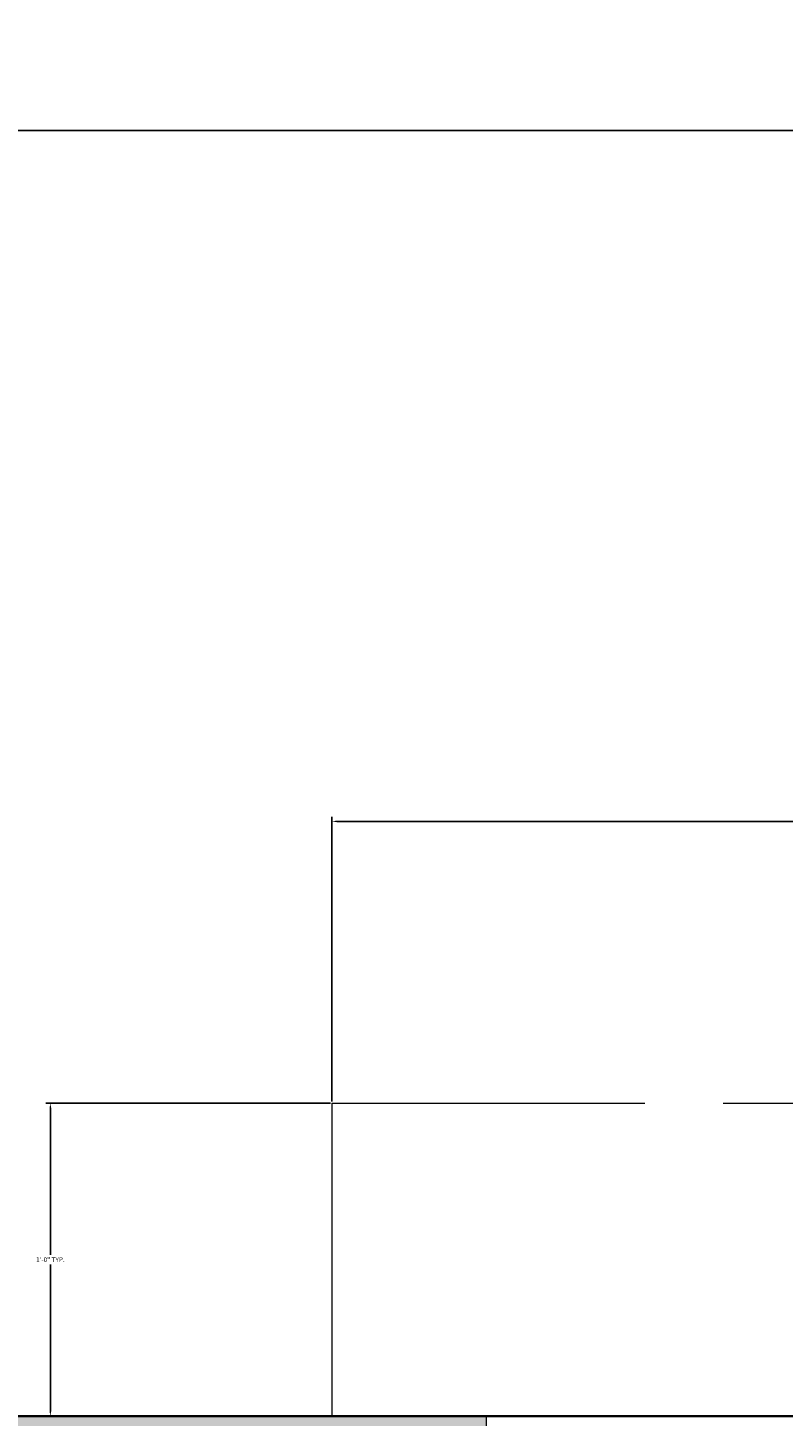
# Model space of a CAD drawing. Units: inches. Extents: x -5 to 482, y -460 to 66.
# Tile 27 of 31: x 48 to 77, y 13 to 66. Entities that reach past the tile are written whole.
import ezdxf

# ---------------------------------------------------------------- set-up
doc = ezdxf.new("R2010")
doc.units = ezdxf.units.IN
doc.header["$MEASUREMENT"] = 0
doc.linetypes.add('ACAD_ISO02W100', pattern=[15, 12, -3])
for name, color, linetype, lineweight in [('A-ANNO-DIMS', 2, 'Continuous', 18), ('A-GLAZ', 4, 'Continuous', 18), ('A-GLAZ-OVHD', 4, 'ACAD_ISO02W100', 13), ('A-WALL', 7, 'Continuous', 35), ('A-WALL-PATT', 152, 'Continuous', 13)]:
    doc.layers.add(name, color=color, linetype=linetype, lineweight=lineweight)
doc.styles.get("Standard").update_dxf_attribs({"font": 'arial.ttf'})
doc.dimstyles.get("Standard").update_dxf_attribs({"dimtxt": 0.18, "dimasz": 0.18, "dimexe": 0.18, "dimexo": 0.0625, "dimgap": 0.09, "dimtad": 0, "dimtih": 1, "dimtoh": 1, "dimdec": 0, "dimzin": 0, "dimdsep": 46, "dimlunit": 3, "dimtxsty": 'Standard', "dimcen": 0.09, "dimadec": 0, "dimazin": 0, "dimtfac": 1, "dimtdec": 0, "dimtofl": 0, "dimtmove": 0, "dimatfit": 3, "dimfxl": 1, "dimtolj": 1, "dimtzin": 0, "dimarcsym": 0})

# ---------------------------------------------------------------- blocks, each defined once
blk = doc.blocks.new('*D3')
at = {"layer": 'A-ANNO-DIMS', "color": 0, "lineweight": -2, "transparency": 16777216}
for p, q in [((32.877, 13.214), (32.877, 62.612)), ((33.057, 62.432), (221.233, 62.432)), ((430.197, 62.432), (242.02, 62.432)), ((430.377, 13.214), (430.377, 62.612))]:
    blk.add_line(p, q, dxfattribs=at)
at = {"layer": 'A-ANNO-DIMS', "color": 0, "transparency": 16777216}
for points in [[(33.057, 62.462), (33.057, 62.402), (32.877, 62.432)], [(430.197, 62.462), (430.197, 62.402), (430.377, 62.432)]]:
    blk.add_solid(points, dxfattribs=at)
at = {"layer": 'Defpoints', "color": 0, "transparency": 16777216}
for p in [(430.377, 62.432), (32.877, 13.151), (430.377, 13.151)]:
    blk.add_point(p, dxfattribs=at)
at = {"layer": 'A-ANNO-DIMS', "color": 0, "transparency": 16777216, "insert": (231.627, 62.432), "char_height": 6, "attachment_point": 5}
blk.add_mtext('\\A1;33\'-2"', dxfattribs=at)
blk = doc.blocks.new('WIN-SHADE-72IN')
for q in [(72, 12), (0, 0)]:
    blk.add_line((0, 12), q)
blk = doc.blocks.new('*D45')
at = {"layer": 'A-ANNO-DIMS', "color": 0, "lineweight": -2, "transparency": 16777216}
for p, q in [((59.948, 25.214), (59.948, 36.131)), ((60.128, 35.951), (94.251, 35.951)), ((131.768, 35.951), (97.645, 35.951)), ((131.948, 25.214), (131.948, 36.131))]:
    blk.add_line(p, q, dxfattribs=at)
at = {"layer": 'A-ANNO-DIMS', "color": 0, "transparency": 16777216}
for points in [[(60.128, 35.981), (60.128, 35.921), (59.948, 35.951)], [(131.768, 35.981), (131.768, 35.921), (131.948, 35.951)]]:
    blk.add_solid(points, dxfattribs=at)
at = {"layer": 'Defpoints', "color": 0, "transparency": 16777216}
for p in [(131.948, 35.951), (59.948, 25.151), (131.948, 25.151)]:
    blk.add_point(p, dxfattribs=at)
at = {"layer": 'A-ANNO-DIMS', "color": 0, "transparency": 16777216, "insert": (95.948, 35.951), "char_height": 0.18, "attachment_point": 5}
blk.add_mtext('\\A1;WINDOW SHADE 6\'-0" TYP.', dxfattribs=at)
blk = doc.blocks.new('*D46')
at = {"layer": 'A-ANNO-DIMS', "color": 0, "lineweight": -2, "transparency": 16777216}
for p, q in [((59.885, 25.151), (48.968, 25.151)), ((49.148, 24.971), (49.148, 19.333)), ((49.148, 13.331), (49.148, 18.969)), ((59.885, 13.151), (48.968, 13.151))]:
    blk.add_line(p, q, dxfattribs=at)
at = {"layer": 'A-ANNO-DIMS', "color": 0, "transparency": 16777216}
for points in [[(49.118, 24.971), (49.178, 24.971), (49.148, 25.151)], [(49.118, 13.331), (49.178, 13.331), (49.148, 13.151)]]:
    blk.add_solid(points, dxfattribs=at)
at = {"layer": 'Defpoints', "color": 0, "transparency": 16777216}
for p in [(49.148, 25.151), (59.948, 25.151), (59.948, 13.151)]:
    blk.add_point(p, dxfattribs=at)
at = {"layer": 'A-ANNO-DIMS', "color": 0, "transparency": 16777216, "insert": (49.148, 19.151), "char_height": 0.18, "attachment_point": 5}
blk.add_mtext('\\A1;1\'-0" TYP.', dxfattribs=at)

msp = doc.modelspace()

# ---------------------------------------------------------------- hatches: boundary and pattern name
at = {"layer": 'A-WALL-PATT'}
h = msp.add_hatch(color=256, dxfattribs=at)
h.dxf.hatch_style = 1
h.paths.add_polyline_path([(149.377, -412.849), (144.377, -412.849), (144.377, -283.849), (144.377, -279.349), (133.877, -279.349), (133.877, -283.849), (139.877, -283.849), (139.877, -412.849), (133.51, -412.849), (133.51, -413.916), (102.652, -413.916), (102.652, -421.02), (133.51, -421.02), (133.51, -421.849), (149.377, -421.849)])
h.paths.add_polyline_path([(226.054, -412.849), (218.877, -412.849), (218.877, -350.849), (262.877, -350.849), (262.877, -386.849), (267.377, -386.849), (267.377, -283.849), (270.377, -283.849), (270.377, -279.349), (244.877, -279.349), (244.877, -283.849), (262.877, -283.849), (262.877, -346.349), (218.877, -346.349), (218.877, -283.849), (220.877, -283.849), (220.877, -279.349), (214.377, -279.349), (214.377, -283.849), (214.377, -412.849), (209.377, -412.849), (209.377, -421.849), (226.054, -421.849)])
h.paths.add_polyline_path([(315.815, -412.849), (250.054, -412.849), (250.054, -421.849), (315.815, -421.849)])
h.paths.add_polyline_path([(430.377, -378.349), (421.377, -378.349), (421.377, -412.849), (375.815, -412.849), (375.815, -421.849), (430.377, -421.849)])
h.paths.add_polyline_path([(78.691, -413.916), (47.68, -413.916), (47.68, -412.849), (41.877, -412.849), (41.877, -283.849), (109.877, -283.849), (109.877, -279.349), (41.877, -279.349), (41.877, -241.849), (32.877, -241.849), (32.877, -421.849), (47.68, -421.849), (47.68, -421.02), (78.691, -421.02)])
h.paths.add_polyline_path([(41.877, -144.349), (154.377, -144.349), (154.377, -137.849), (149.877, -137.849), (149.877, -139.849), (41.877, -139.849), (41.877, -97.849), (32.877, -97.849), (32.877, -181.849), (41.877, -181.849)])
h.paths.add_polyline_path([(430.377, -241.849), (421.377, -241.849), (421.377, -279.349), (309.377, -279.349), (309.377, -170.349), (304.877, -170.349), (304.877, -279.349), (294.377, -279.349), (294.377, -283.849), (421.377, -283.849), (421.377, -318.349), (430.377, -318.349)])
h.paths.add_polyline_path([(430.377, -119.849), (421.377, -119.849), (421.377, -139.849), (419.377, -139.849), (419.377, -144.349), (421.377, -144.349), (421.377, -181.849), (430.377, -181.849)])
h.paths.add_polyline_path([(395.377, -139.849), (377.377, -139.849), (377.377, -75.849), (421.377, -75.849), (421.377, -95.849), (430.377, -95.849), (430.377, -45.599), (421.377, -45.599), (421.377, -71.349), (377.377, -71.349), (377.377, -22.849), (372.877, -22.849), (372.877, -139.849), (242.877, -139.849), (242.877, -137.849), (238.377, -137.849), (238.377, -144.349), (304.877, -144.349), (304.877, -146.349), (309.377, -146.349), (309.377, -144.349), (395.377, -144.349)])
h.paths.add_polyline_path([(65.877, 13.151), (32.877, 13.151), (32.877, -37.849), (41.877, -37.849), (41.877, 4.151), (65.877, 4.151)])
h.paths.add_polyline_path([(166.377, 13.151), (125.877, 13.151), (125.877, 4.151), (149.877, 4.151), (149.877, -113.849), (154.377, -113.849), (154.377, 4.151), (166.377, 4.151)])
h.paths.add_polyline_path([(277.877, 13.151), (226.377, 13.151), (226.377, 4.151), (238.377, 4.151), (238.377, -113.849), (242.877, -113.849), (242.877, 4.151), (277.877, 4.151)])
h.paths.add_polyline_path([(430.377, 13.151), (337.877, 13.151), (337.877, 4.151), (372.877, 4.151), (372.877, 1.151), (377.377, 1.151), (377.377, 4.151), (421.377, 4.151), (421.377, -21.599), (430.377, -21.599)])

# ---------------------------------------------------------------- linework, layer by layer
at = {"layer": 'A-GLAZ'}
msp.add_line((65.877, 4.151), (65.877, 13.151), dxfattribs=at)
at = {"layer": 'A-WALL'}
msp.add_line((32.877, 13.151), (430.377, 13.151), dxfattribs=at)

# ---------------------------------------------------------------- block references
at = {"layer": 'A-GLAZ-OVHD'}
msp.add_blockref('WIN-SHADE-72IN', (59.948, 13.151), dxfattribs=at)

# ---------------------------------------------------------------- dimensions: what is measured, and where the dimension line sits
at = {"layer": 'A-ANNO-DIMS'}
dim = msp.add_linear_dim(base=(430.376735986, 62.431571932), p1=(32.876735986, 13.151335974), p2=(430.376735986, 13.151335974), dimstyle='Standard', override={"dimtxt": 6, "dimclrd": 0, "dimclre": 0, "dimclrt": 0}, dxfattribs=at)
dim.commit()
dim.dimension.update_dxf_attribs({"geometry": '*D3', "text_midpoint": (231.626735986, 62.431571932)})
dim = msp.add_linear_dim(base=(131.948, 35.951), p1=(59.948, 25.151), p2=(131.948, 25.151), text='WINDOW SHADE <> TYP.', dimstyle='Standard', override={"dimdec": 1, "dimlfac": 1, "dimrnd": 0, "dimzin": 1, "dimdsep": 46, "dimlunit": 4, "dimfrac": 2}, dxfattribs=at)
dim.commit()
dim.dimension.update_dxf_attribs({"geometry": '*D45', "text_midpoint": (95.948, 35.951)})
dim = msp.add_linear_dim(base=(49.148, 25.151), p1=(59.948, 13.151), p2=(59.948, 25.151), angle=90, text='<> TYP.', dimstyle='Standard', override={"dimdec": 1, "dimlfac": 1, "dimrnd": 0, "dimzin": 1, "dimdsep": 46, "dimlunit": 4, "dimfrac": 2}, dxfattribs=at)
dim.commit()
dim.dimension.update_dxf_attribs({"geometry": '*D46', "text_midpoint": (49.148, 19.151)})

doc.saveas('drawing.dxf')
